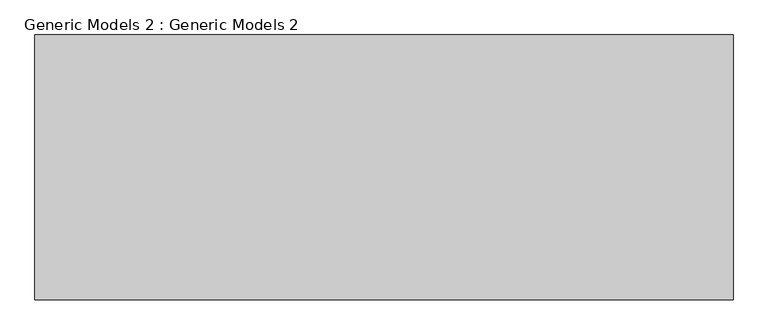
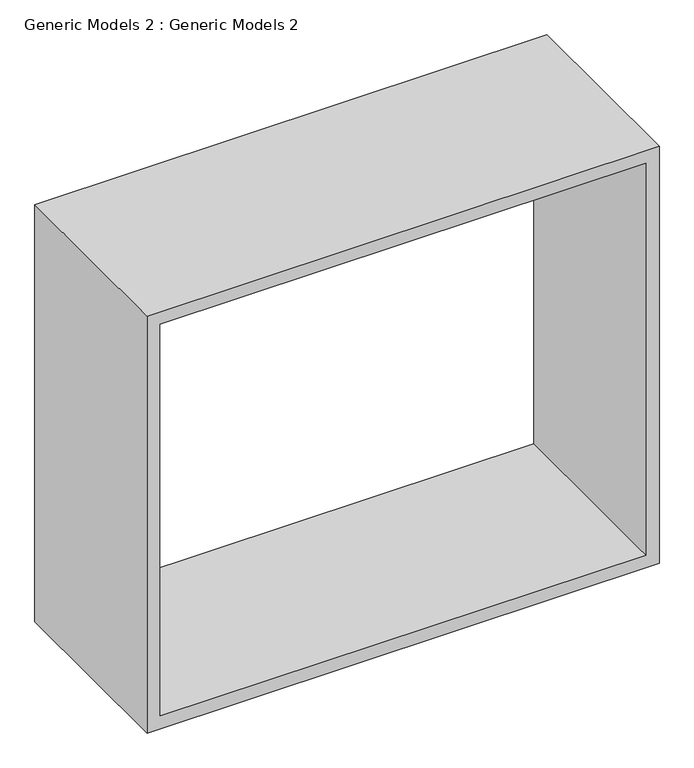
"""IFC4 building model written with IfcOpenShell, lengths in millimetres: proxy geometry, Generic Models 2 : Generic Models 2."""

from ifc_helpers import new_model, si_unit, frame, origin, place, context, project, spatial, polyline, outline, extrude, source, transform, mapped, element, save


def generic_models_2_generic_models_2_0bdea63f(model_context):
    return source(origin(), model_context, "Body", "SweptSolid", [
        extrude(outline(polyline([(9310.258551, 675.4218735), (9310.258551, -6131.7781265), (3454.1550828, -6131.7781265), (3454.1550828, 675.4218735), (9310.258551, 675.4218735)]), holes=[polyline([(9132.458551, 497.6218735), (3631.9550828, 497.6218735), (3631.9550828, -5953.9781265), (9132.458551, -5953.9781265), (9132.458551, 497.6218735)])]), frame((0.0, -6969.5291288, 0.0), z_axis=(0.0, 1.0, 0.0), x_axis=(0.0, 0.0, 1.0)), (0.0, 0.0, 1.0), 2580.3148756),
    ])


if __name__ == "__main__":
    model = new_model("IFC4")
    model_context = context("Model", 3, world=origin())
    ifc_project = project(units=[si_unit("LENGTHUNIT", "METRE", prefix="MILLI")], contexts=[model_context])
    site = spatial("IfcSite", under=ifc_project)
    building = spatial("IfcBuilding", under=site)
    placement = place(None, origin())
    generic_models_2_generic_models_2_shape = generic_models_2_generic_models_2_0bdea63f(model_context)
    element("IfcBuildingElementProxy", 1, Name="Generic Models 2 : Generic Models 2", ObjectType="Generic Models 2 : Generic Models 2", at=placement, inside=building, context=model_context, shape_type="MappedRepresentation", body=[
        mapped(generic_models_2_generic_models_2_shape, transform((0.0, 0.0, 0.0), x_axis=(1.0, 0.0, 0.0), y_axis=(0.0, 1.0, 0.0), z_axis=(0.0, 0.0, 1.0))),
    ])
    save(model, "model.ifc")
